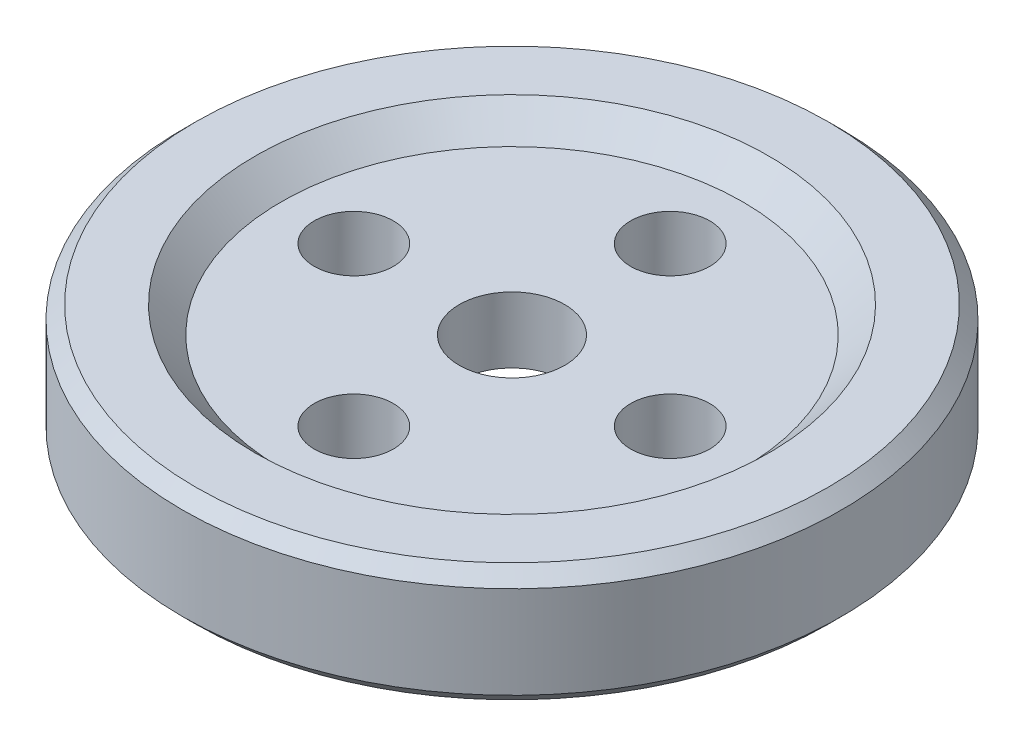
ISO-10303-21;
HEADER;
FILE_DESCRIPTION(('STEP AP214'),'2;1');
FILE_NAME('part.step','',(''),(''),'','','');
FILE_SCHEMA(('AUTOMOTIVE_DESIGN { 1 0 10303 214 1 1 1 1 }'));
ENDSEC;
DATA;
#1=APPLICATION_CONTEXT('core data for automotive mechanical design processes');
#2=APPLICATION_PROTOCOL_DEFINITION('international standard','automotive_design',2000,#1);
#3=PRODUCT_CONTEXT('',#1,'mechanical');
#4=PRODUCT('Part','Part','',(#3));
#5=PRODUCT_RELATED_PRODUCT_CATEGORY('part','',(#4));
#6=PRODUCT_DEFINITION_FORMATION('','',#4);
#7=PRODUCT_DEFINITION_CONTEXT('part definition',#1,'design');
#8=PRODUCT_DEFINITION('design','',#6,#7);
#9=PRODUCT_DEFINITION_SHAPE('','',#8);
#10=(LENGTH_UNIT() NAMED_UNIT(*) SI_UNIT(.MILLI.,.METRE.));
#11=(NAMED_UNIT(*) PLANE_ANGLE_UNIT() SI_UNIT($,.RADIAN.));
#12=(NAMED_UNIT(*) SI_UNIT($,.STERADIAN.) SOLID_ANGLE_UNIT());
#13=UNCERTAINTY_MEASURE_WITH_UNIT(LENGTH_MEASURE(1.E-05),#10,'distance_accuracy_value','');
#14=(GEOMETRIC_REPRESENTATION_CONTEXT(3) GLOBAL_UNCERTAINTY_ASSIGNED_CONTEXT((#13)) GLOBAL_UNIT_ASSIGNED_CONTEXT((#10,
#11,#12)) REPRESENTATION_CONTEXT('',''));
#15=CARTESIAN_POINT('',(0.,0.,0.));
#16=DIRECTION('',(0.,0.,1.));
#17=DIRECTION('',(1.,0.,0.));
#18=AXIS2_PLACEMENT_3D('',#15,#16,#17);
#19=CARTESIAN_POINT('',(0.,4.5,0.));
#20=DIRECTION('',(0.,-1.,0.));
#21=DIRECTION('',(0.,0.,-1.));
#22=AXIS2_PLACEMENT_3D('',#19,#20,#21);
#23=CYLINDRICAL_SURFACE('',#22,25.);
#24=CARTESIAN_POINT('',(0.,-3.5,0.));
#25=DIRECTION('',(0.,1.,0.));
#26=DIRECTION('',(0.,0.,1.));
#27=AXIS2_PLACEMENT_3D('',#24,#25,#26);
#28=CIRCLE('',#27,25.);
#29=CARTESIAN_POINT('',(0.,-3.5,25.));
#30=VERTEX_POINT('',#29);
#31=EDGE_CURVE('E62',#30,#30,#28,.T.);
#32=ORIENTED_EDGE('',*,*,#31,.T.);
#33=EDGE_LOOP('',(#32));
#34=FACE_BOUND('',#33,.T.);
#35=CARTESIAN_POINT('',(0.,3.5,0.));
#36=DIRECTION('',(0.,1.,0.));
#37=DIRECTION('',(0.,0.,1.));
#38=AXIS2_PLACEMENT_3D('',#35,#36,#37);
#39=CIRCLE('',#38,25.);
#40=CARTESIAN_POINT('',(0.,3.5,25.));
#41=VERTEX_POINT('',#40);
#42=EDGE_CURVE('E68',#41,#41,#39,.F.);
#43=ORIENTED_EDGE('',*,*,#42,.T.);
#44=EDGE_LOOP('',(#43));
#45=FACE_BOUND('',#44,.T.);
#46=ADVANCED_FACE('F44',(#34,#45),#23,.T.);
#47=CARTESIAN_POINT('',(0.,4.5,0.));
#48=DIRECTION('',(0.,1.,0.));
#49=DIRECTION('',(0.,0.,1.));
#50=AXIS2_PLACEMENT_3D('',#47,#48,#49);
#51=PLANE('',#50);
#52=CARTESIAN_POINT('',(0.,4.5,0.));
#53=DIRECTION('',(0.,1.,0.));
#54=DIRECTION('',(0.,0.,1.));
#55=AXIS2_PLACEMENT_3D('',#52,#53,#54);
#56=CIRCLE('',#55,24.);
#57=CARTESIAN_POINT('',(0.,4.5,24.));
#58=VERTEX_POINT('',#57);
#59=EDGE_CURVE('E67',#58,#58,#56,.T.);
#60=ORIENTED_EDGE('',*,*,#59,.T.);
#61=EDGE_LOOP('',(#60));
#62=FACE_BOUND('',#61,.T.);
#63=CARTESIAN_POINT('',(0.,4.5,0.));
#64=DIRECTION('',(0.,1.,0.));
#65=DIRECTION('',(0.,0.,1.));
#66=AXIS2_PLACEMENT_3D('',#63,#64,#65);
#67=CIRCLE('',#66,19.5);
#68=CARTESIAN_POINT('',(0.,4.5,19.5));
#69=VERTEX_POINT('',#68);
#70=EDGE_CURVE('E75',#69,#69,#67,.F.);
#71=ORIENTED_EDGE('',*,*,#70,.T.);
#72=EDGE_LOOP('',(#71));
#73=FACE_BOUND('',#72,.T.);
#74=ADVANCED_FACE('F137',(#62,#73),#51,.T.);
#75=CARTESIAN_POINT('',(0.,-4.5,0.));
#76=DIRECTION('',(0.,1.,0.));
#77=DIRECTION('',(0.,0.,1.));
#78=AXIS2_PLACEMENT_3D('',#75,#76,#77);
#79=PLANE('',#78);
#80=CARTESIAN_POINT('',(0.,-4.5,0.));
#81=DIRECTION('',(0.,1.,0.));
#82=DIRECTION('',(0.,0.,1.));
#83=AXIS2_PLACEMENT_3D('',#80,#81,#82);
#84=CIRCLE('',#83,19.5);
#85=CARTESIAN_POINT('',(0.,-4.5,19.5));
#86=VERTEX_POINT('',#85);
#87=EDGE_CURVE('E10',#86,#86,#84,.T.);
#88=ORIENTED_EDGE('',*,*,#87,.T.);
#89=EDGE_LOOP('',(#88));
#90=FACE_BOUND('',#89,.T.);
#91=CARTESIAN_POINT('',(0.,-4.5,0.));
#92=DIRECTION('',(0.,1.,0.));
#93=DIRECTION('',(0.,0.,1.));
#94=AXIS2_PLACEMENT_3D('',#91,#92,#93);
#95=CIRCLE('',#94,24.);
#96=CARTESIAN_POINT('',(0.,-4.5,24.));
#97=VERTEX_POINT('',#96);
#98=EDGE_CURVE('E60',#97,#97,#95,.F.);
#99=ORIENTED_EDGE('',*,*,#98,.T.);
#100=EDGE_LOOP('',(#99));
#101=FACE_BOUND('',#100,.T.);
#102=ADVANCED_FACE('F113',(#90,#101),#79,.F.);
#103=CARTESIAN_POINT('',(0.,2.5,0.));
#104=DIRECTION('',(0.,1.,0.));
#105=DIRECTION('',(0.,0.,1.));
#106=AXIS2_PLACEMENT_3D('',#103,#104,#105);
#107=PLANE('',#106);
#108=CARTESIAN_POINT('',(0.,2.5,0.));
#109=DIRECTION('',(0.,1.,0.));
#110=DIRECTION('',(0.,0.,1.));
#111=AXIS2_PLACEMENT_3D('',#108,#109,#110);
#112=CIRCLE('',#111,17.5);
#113=CARTESIAN_POINT('',(0.,2.5,17.5));
#114=VERTEX_POINT('',#113);
#115=EDGE_CURVE('E73',#114,#114,#112,.T.);
#116=ORIENTED_EDGE('',*,*,#115,.T.);
#117=EDGE_LOOP('',(#116));
#118=FACE_BOUND('',#117,.T.);
#119=CARTESIAN_POINT('',(0.,2.5,0.));
#120=DIRECTION('',(0.,1.,0.));
#121=DIRECTION('',(0.,0.,1.));
#122=AXIS2_PLACEMENT_3D('',#119,#120,#121);
#123=CIRCLE('',#122,4.);
#124=CARTESIAN_POINT('',(0.,2.5,4.));
#125=VERTEX_POINT('',#124);
#126=EDGE_CURVE('E101',#125,#125,#123,.T.);
#127=ORIENTED_EDGE('',*,*,#126,.F.);
#128=EDGE_LOOP('',(#127));
#129=FACE_BOUND('',#128,.T.);
#130=CARTESIAN_POINT('',(0.,2.5,-12.));
#131=DIRECTION('',(0.,1.,0.));
#132=DIRECTION('',(0.,0.,1.));
#133=AXIS2_PLACEMENT_3D('',#130,#131,#132);
#134=CIRCLE('',#133,3.);
#135=CARTESIAN_POINT('',(0.,2.5,-9.));
#136=VERTEX_POINT('',#135);
#137=EDGE_CURVE('E91',#136,#136,#134,.T.);
#138=ORIENTED_EDGE('',*,*,#137,.F.);
#139=EDGE_LOOP('',(#138));
#140=FACE_BOUND('',#139,.T.);
#141=CARTESIAN_POINT('',(-12.,2.5,0.));
#142=DIRECTION('',(0.,1.,0.));
#143=DIRECTION('',(0.,0.,1.));
#144=AXIS2_PLACEMENT_3D('',#141,#142,#143);
#145=CIRCLE('',#144,3.);
#146=CARTESIAN_POINT('',(-12.,2.5,3.));
#147=VERTEX_POINT('',#146);
#148=EDGE_CURVE('E98',#147,#147,#145,.T.);
#149=ORIENTED_EDGE('',*,*,#148,.F.);
#150=EDGE_LOOP('',(#149));
#151=FACE_BOUND('',#150,.T.);
#152=CARTESIAN_POINT('',(0.,2.5,12.));
#153=DIRECTION('',(0.,1.,0.));
#154=DIRECTION('',(0.,0.,1.));
#155=AXIS2_PLACEMENT_3D('',#152,#153,#154);
#156=CIRCLE('',#155,3.);
#157=CARTESIAN_POINT('',(0.,2.5,15.));
#158=VERTEX_POINT('',#157);
#159=EDGE_CURVE('E94',#158,#158,#156,.T.);
#160=ORIENTED_EDGE('',*,*,#159,.F.);
#161=EDGE_LOOP('',(#160));
#162=FACE_BOUND('',#161,.T.);
#163=CARTESIAN_POINT('',(12.,2.5,0.));
#164=DIRECTION('',(0.,1.,0.));
#165=DIRECTION('',(0.,0.,1.));
#166=AXIS2_PLACEMENT_3D('',#163,#164,#165);
#167=CIRCLE('',#166,3.);
#168=CARTESIAN_POINT('',(12.,2.5,3.));
#169=VERTEX_POINT('',#168);
#170=EDGE_CURVE('E100',#169,#169,#167,.T.);
#171=ORIENTED_EDGE('',*,*,#170,.F.);
#172=EDGE_LOOP('',(#171));
#173=FACE_BOUND('',#172,.T.);
#174=ADVANCED_FACE('F112',(#118,#129,#140,#151,#162,#173),#107,.T.);
#175=CARTESIAN_POINT('',(0.,-2.5,0.));
#176=DIRECTION('',(0.,-1.,0.));
#177=DIRECTION('',(0.,0.,-1.));
#178=AXIS2_PLACEMENT_3D('',#175,#176,#177);
#179=PLANE('',#178);
#180=CARTESIAN_POINT('',(0.,-2.5,0.));
#181=DIRECTION('',(0.,-1.,0.));
#182=DIRECTION('',(0.,0.,-1.));
#183=AXIS2_PLACEMENT_3D('',#180,#181,#182);
#184=CIRCLE('',#183,17.5);
#185=CARTESIAN_POINT('',(0.,-2.5,-17.5));
#186=VERTEX_POINT('',#185);
#187=EDGE_CURVE('E52',#186,#186,#184,.T.);
#188=ORIENTED_EDGE('',*,*,#187,.T.);
#189=EDGE_LOOP('',(#188));
#190=FACE_BOUND('',#189,.T.);
#191=CARTESIAN_POINT('',(0.,-2.5,-12.));
#192=DIRECTION('',(0.,-1.,0.));
#193=DIRECTION('',(0.,0.,-1.));
#194=AXIS2_PLACEMENT_3D('',#191,#192,#193);
#195=CIRCLE('',#194,3.);
#196=CARTESIAN_POINT('',(0.,-2.5,-15.));
#197=VERTEX_POINT('',#196);
#198=EDGE_CURVE('E80',#197,#197,#195,.T.);
#199=ORIENTED_EDGE('',*,*,#198,.F.);
#200=EDGE_LOOP('',(#199));
#201=FACE_BOUND('',#200,.T.);
#202=CARTESIAN_POINT('',(0.,-2.5,0.));
#203=DIRECTION('',(0.,-1.,0.));
#204=DIRECTION('',(0.,0.,-1.));
#205=AXIS2_PLACEMENT_3D('',#202,#203,#204);
#206=CIRCLE('',#205,4.);
#207=CARTESIAN_POINT('',(0.,-2.5,-4.));
#208=VERTEX_POINT('',#207);
#209=EDGE_CURVE('E83',#208,#208,#206,.T.);
#210=ORIENTED_EDGE('',*,*,#209,.F.);
#211=EDGE_LOOP('',(#210));
#212=FACE_BOUND('',#211,.T.);
#213=CARTESIAN_POINT('',(-12.,-2.5,0.));
#214=DIRECTION('',(0.,-1.,0.));
#215=DIRECTION('',(0.,0.,-1.));
#216=AXIS2_PLACEMENT_3D('',#213,#214,#215);
#217=CIRCLE('',#216,3.);
#218=CARTESIAN_POINT('',(-12.,-2.5,-3.));
#219=VERTEX_POINT('',#218);
#220=EDGE_CURVE('E82',#219,#219,#217,.T.);
#221=ORIENTED_EDGE('',*,*,#220,.F.);
#222=EDGE_LOOP('',(#221));
#223=FACE_BOUND('',#222,.T.);
#224=CARTESIAN_POINT('',(0.,-2.5,12.));
#225=DIRECTION('',(0.,-1.,0.));
#226=DIRECTION('',(0.,0.,-1.));
#227=AXIS2_PLACEMENT_3D('',#224,#225,#226);
#228=CIRCLE('',#227,3.);
#229=CARTESIAN_POINT('',(0.,-2.5,9.));
#230=VERTEX_POINT('',#229);
#231=EDGE_CURVE('E87',#230,#230,#228,.T.);
#232=ORIENTED_EDGE('',*,*,#231,.F.);
#233=EDGE_LOOP('',(#232));
#234=FACE_BOUND('',#233,.T.);
#235=CARTESIAN_POINT('',(12.,-2.5,0.));
#236=DIRECTION('',(0.,-1.,0.));
#237=DIRECTION('',(0.,0.,-1.));
#238=AXIS2_PLACEMENT_3D('',#235,#236,#237);
#239=CIRCLE('',#238,3.);
#240=CARTESIAN_POINT('',(12.,-2.5,-3.));
#241=VERTEX_POINT('',#240);
#242=EDGE_CURVE('E89',#241,#241,#239,.T.);
#243=ORIENTED_EDGE('',*,*,#242,.F.);
#244=EDGE_LOOP('',(#243));
#245=FACE_BOUND('',#244,.T.);
#246=ADVANCED_FACE('F111',(#190,#201,#212,#223,#234,#245),#179,.T.);
#247=CARTESIAN_POINT('',(12.,-81.5,0.));
#248=DIRECTION('',(0.,1.,0.));
#249=DIRECTION('',(0.,0.,1.));
#250=AXIS2_PLACEMENT_3D('',#247,#248,#249);
#251=CYLINDRICAL_SURFACE('',#250,3.);
#252=ORIENTED_EDGE('',*,*,#242,.T.);
#253=EDGE_LOOP('',(#252));
#254=FACE_BOUND('',#253,.T.);
#255=ORIENTED_EDGE('',*,*,#170,.T.);
#256=EDGE_LOOP('',(#255));
#257=FACE_BOUND('',#256,.T.);
#258=ADVANCED_FACE('F122',(#254,#257),#251,.F.);
#259=CARTESIAN_POINT('',(0.,-81.5,12.));
#260=DIRECTION('',(0.,1.,0.));
#261=DIRECTION('',(0.,0.,1.));
#262=AXIS2_PLACEMENT_3D('',#259,#260,#261);
#263=CYLINDRICAL_SURFACE('',#262,3.);
#264=ORIENTED_EDGE('',*,*,#231,.T.);
#265=EDGE_LOOP('',(#264));
#266=FACE_BOUND('',#265,.T.);
#267=ORIENTED_EDGE('',*,*,#159,.T.);
#268=EDGE_LOOP('',(#267));
#269=FACE_BOUND('',#268,.T.);
#270=ADVANCED_FACE('F127',(#266,#269),#263,.F.);
#271=CARTESIAN_POINT('',(-12.,-81.5,0.));
#272=DIRECTION('',(0.,1.,0.));
#273=DIRECTION('',(0.,0.,1.));
#274=AXIS2_PLACEMENT_3D('',#271,#272,#273);
#275=CYLINDRICAL_SURFACE('',#274,3.);
#276=ORIENTED_EDGE('',*,*,#220,.T.);
#277=EDGE_LOOP('',(#276));
#278=FACE_BOUND('',#277,.T.);
#279=ORIENTED_EDGE('',*,*,#148,.T.);
#280=EDGE_LOOP('',(#279));
#281=FACE_BOUND('',#280,.T.);
#282=ADVANCED_FACE('F135',(#278,#281),#275,.F.);
#283=CARTESIAN_POINT('',(0.,-81.5,0.));
#284=DIRECTION('',(0.,1.,0.));
#285=DIRECTION('',(0.,0.,1.));
#286=AXIS2_PLACEMENT_3D('',#283,#284,#285);
#287=CYLINDRICAL_SURFACE('',#286,4.);
#288=ORIENTED_EDGE('',*,*,#209,.T.);
#289=EDGE_LOOP('',(#288));
#290=FACE_BOUND('',#289,.T.);
#291=ORIENTED_EDGE('',*,*,#126,.T.);
#292=EDGE_LOOP('',(#291));
#293=FACE_BOUND('',#292,.T.);
#294=ADVANCED_FACE('F211',(#290,#293),#287,.F.);
#295=CARTESIAN_POINT('',(0.,-81.5,-12.));
#296=DIRECTION('',(0.,1.,0.));
#297=DIRECTION('',(0.,0.,1.));
#298=AXIS2_PLACEMENT_3D('',#295,#296,#297);
#299=CYLINDRICAL_SURFACE('',#298,3.);
#300=ORIENTED_EDGE('',*,*,#198,.T.);
#301=EDGE_LOOP('',(#300));
#302=FACE_BOUND('',#301,.T.);
#303=ORIENTED_EDGE('',*,*,#137,.T.);
#304=EDGE_LOOP('',(#303));
#305=FACE_BOUND('',#304,.T.);
#306=ADVANCED_FACE('F108',(#302,#305),#299,.F.);
#307=CARTESIAN_POINT('',(0.,2.5,0.));
#308=DIRECTION('',(0.,1.,0.));
#309=DIRECTION('',(0.,0.,1.));
#310=AXIS2_PLACEMENT_3D('',#307,#308,#309);
#311=CONICAL_SURFACE('',#310,17.5,0.785398163397453);
#312=ORIENTED_EDGE('',*,*,#70,.F.);
#313=EDGE_LOOP('',(#312));
#314=FACE_BOUND('',#313,.T.);
#315=ORIENTED_EDGE('',*,*,#115,.F.);
#316=EDGE_LOOP('',(#315));
#317=FACE_BOUND('',#316,.T.);
#318=ADVANCED_FACE('F151',(#314,#317),#311,.F.);
#319=CARTESIAN_POINT('',(0.,4.5,0.));
#320=DIRECTION('',(0.,-1.,0.));
#321=DIRECTION('',(0.,0.,-1.));
#322=AXIS2_PLACEMENT_3D('',#319,#320,#321);
#323=CONICAL_SURFACE('',#322,24.,0.785398163397447);
#324=ORIENTED_EDGE('',*,*,#42,.F.);
#325=EDGE_LOOP('',(#324));
#326=FACE_BOUND('',#325,.T.);
#327=ORIENTED_EDGE('',*,*,#59,.F.);
#328=EDGE_LOOP('',(#327));
#329=FACE_BOUND('',#328,.T.);
#330=ADVANCED_FACE('F160',(#326,#329),#323,.T.);
#331=CARTESIAN_POINT('',(0.,-3.5,0.));
#332=DIRECTION('',(0.,1.,0.));
#333=DIRECTION('',(0.,0.,1.));
#334=AXIS2_PLACEMENT_3D('',#331,#332,#333);
#335=CONICAL_SURFACE('',#334,25.,0.78539816339745);
#336=ORIENTED_EDGE('',*,*,#98,.F.);
#337=EDGE_LOOP('',(#336));
#338=FACE_BOUND('',#337,.T.);
#339=ORIENTED_EDGE('',*,*,#31,.F.);
#340=EDGE_LOOP('',(#339));
#341=FACE_BOUND('',#340,.T.);
#342=ADVANCED_FACE('F162',(#338,#341),#335,.T.);
#343=CARTESIAN_POINT('',(0.,-2.5,0.));
#344=DIRECTION('',(0.,-1.,0.));
#345=DIRECTION('',(0.,0.,-1.));
#346=AXIS2_PLACEMENT_3D('',#343,#344,#345);
#347=CONICAL_SURFACE('',#346,17.5,0.785398163397453);
#348=ORIENTED_EDGE('',*,*,#87,.F.);
#349=EDGE_LOOP('',(#348));
#350=FACE_BOUND('',#349,.T.);
#351=ORIENTED_EDGE('',*,*,#187,.F.);
#352=EDGE_LOOP('',(#351));
#353=FACE_BOUND('',#352,.T.);
#354=ADVANCED_FACE('F48',(#350,#353),#347,.F.);
#355=CLOSED_SHELL('',(#46,#74,#102,#174,#246,#258,#270,#282,#294,#306,#318,#330,#342,#354));
#356=MANIFOLD_SOLID_BREP('B2',#355);
#357=ADVANCED_BREP_SHAPE_REPRESENTATION('',(#18,#356),#14);
#358=SHAPE_DEFINITION_REPRESENTATION(#9,#357);
ENDSEC;
END-ISO-10303-21;
